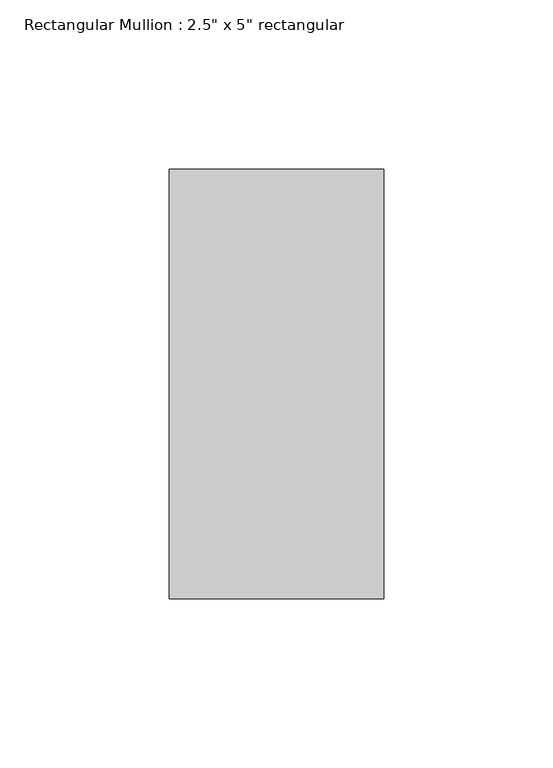
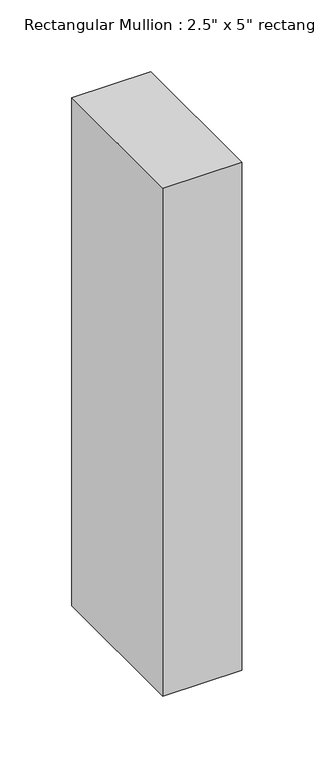
"""IFC4 building model written with IfcOpenShell, lengths in millimetres: member geometry."""

from ifc_helpers import new_model, si_unit, frame, origin, place, context, project, spatial, polyline, outline, extrude, source, transform, mapped, element, save


def member_69a911c1(model_context):
    return source(origin(), model_context, "Body", "SweptSolid", [
        extrude(outline(polyline([(0.0, 63.5), (0.0, -63.5), (-63.5, -63.5), (-63.5, 63.5), (0.0, 63.5)])), frame((0.0, 0.0, -431.8), z_axis=(0.0, 0.0, 1.0), x_axis=(1.0, 0.0, 0.0)), (0.0, 0.0, 1.0), 431.8),
    ])


if __name__ == "__main__":
    model = new_model("IFC4")
    model_context = context("Model", 3, world=origin())
    ifc_project = project(units=[si_unit("LENGTHUNIT", "METRE", prefix="MILLI")], contexts=[model_context])
    site = spatial("IfcSite", under=ifc_project)
    building = spatial("IfcBuilding", under=site)
    placement = place(None, origin())
    member_shape = member_69a911c1(model_context)
    element("IfcMember", 1, ObjectType="Rectangular Mullion : 2.5\" x 5\" rectangular", at=placement, inside=building, context=model_context, shape_type="MappedRepresentation", body=[
        mapped(member_shape, transform((0.0, 0.0, 0.0), x_axis=(1.0, 0.0, 0.0), y_axis=(0.0, 1.0, 0.0), z_axis=(0.0, 0.0, 1.0))),
    ])
    save(model, "model.ifc")

# Revit data of these elements
# Type "Rectangular Mullion : 2.5\" x 5\" rectangular"
#   built-in parameter 1007304 = 0.416667 (stored number, unit not read)
#   built-in parameter 1007301 = 0.104167 (stored number, unit not read)
#   built-in parameter 1007300 = 0.104167 (stored number, unit not read)
# Element 1 (IfcMember, "Rectangular Mullion : 2.5\" x 5\" rectangular")
#   Materials on its faces: "Aluminum"
# Materials
#   "Aluminum": class "Metal", colour RGB 247 247 247, transparency 0, Description = "Aluminum 6061", Cost = 0
